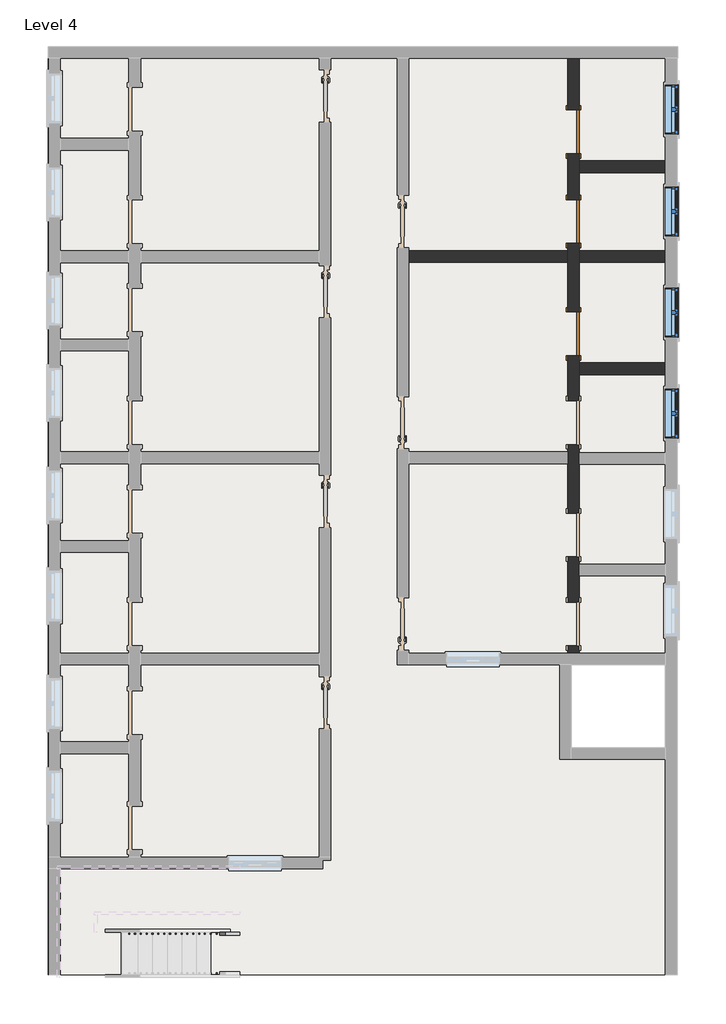
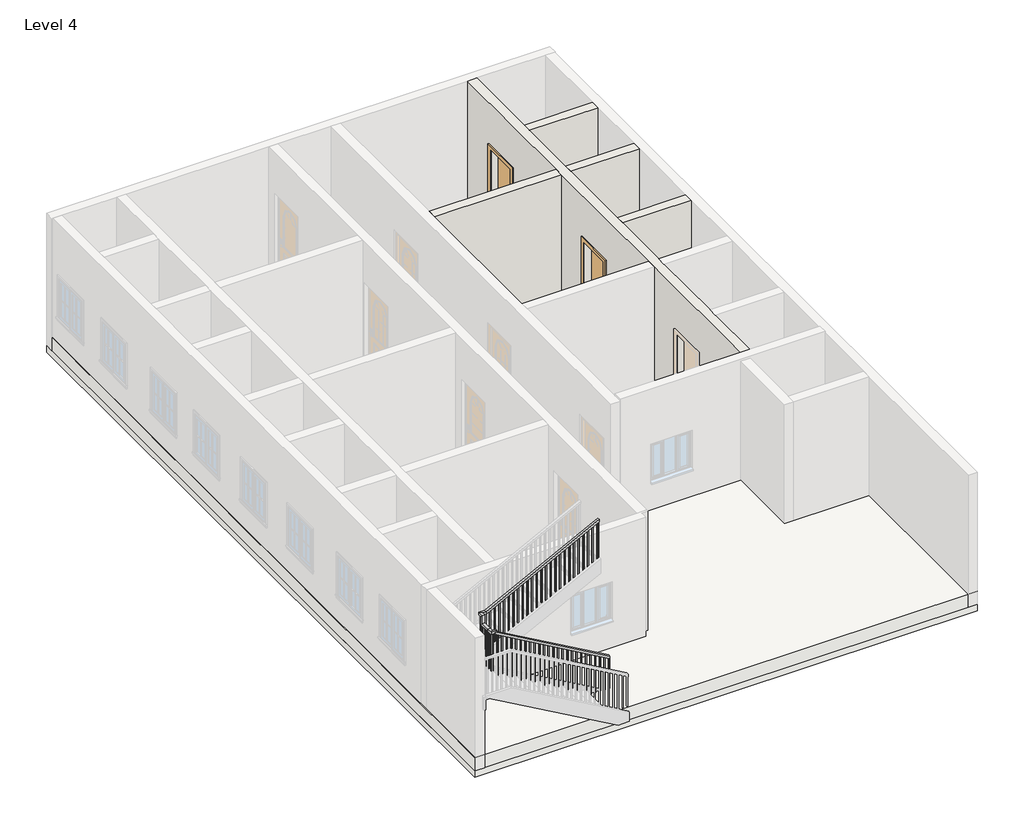
# One storey, part 2 of 4: 5 walls, 4 windows, 3 doors, 1 railing, 1 roof, 1 slab.
"""IFC4 building model written with IfcOpenShell, lengths in millimetres."""

from ifc_helpers import new_model, si_unit, frame, origin, place, context, project, spatial, polyline, outline, extrude, faceted_brep, transform, mapped, element, save
from components import door_53b1b562, window_c29befe5

model = new_model("IFC4")

# Units and contexts
model_context = context("Model", 3, world=origin())
ifc_project = project(units=[si_unit("LENGTHUNIT", "METRE", prefix="MILLI")], contexts=[model_context])

# Site, building, storey
site = spatial("IfcSite", under=ifc_project)
building = spatial("IfcBuilding", under=site)
storey = spatial("IfcBuildingStorey", under=building, Name="Level 4", Elevation=9144.0)

# Doors
placement = place(None, origin())
door_shape = door_53b1b562(model_context)
element("IfcDoor", 1, ObjectType="Single-Flush : 30\" x 80\"", at=placement, inside=storey, context=model_context, shape_type="MappedRepresentation", body=[
    mapped(door_shape, transform((2695.5891134, 6512.9399728, 9144.0), x_axis=(0.0, 1.0, 0.0), y_axis=(-1.0, 0.0, 0.0), z_axis=(0.0, 0.0, 1.0))),
])
element("IfcDoor", 2, ObjectType="Single-Flush : 30\" x 80\"", at=placement, inside=storey, context=model_context, shape_type="MappedRepresentation", body=[
    mapped(door_shape, transform((2695.5891134, 4950.8399728, 9144.0), x_axis=(0.0, 1.0, 0.0), y_axis=(-1.0, 0.0, 0.0), z_axis=(0.0, 0.0, 1.0))),
])
element("IfcDoor", 3, ObjectType="Single-Flush : 30\" x 80\"", at=placement, inside=storey, context=model_context, shape_type="MappedRepresentation", body=[
    mapped(door_shape, transform((2695.5891134, 2995.0399728, 9144.0), x_axis=(0.0, 1.0, 0.0), y_axis=(-1.0, 0.0, 0.0), z_axis=(0.0, 0.0, 1.0))),
])

# Railing
element("IfcRailing", 4, ObjectType="Handrail - Rectangular", at=placement, inside=storey, context=model_context, shape_type="SolidModel", body=[
    faceted_brep([(-3117.2664982, -7482.4600272, 10203.5428571), (-3117.2664982, -7482.4600272, 10145.0339009), (-3117.2664982, -7431.6600272, 10145.0339009), (-3117.2664982, -7431.6600272, 10203.5428571), (-5581.0664982, -7482.4600272, 11611.4285714), (-5631.8664982, -7482.4600272, 11581.9481866), (-5631.8664982, -7431.6600272, 11581.9481866), (-5581.0664982, -7431.6600272, 11611.4285714), (-5581.0664982, -7482.4600272, 11654.9714286), (-5631.8664982, -7482.4600272, 11604.1714286), (-5631.8664982, -7431.6600272, 11604.1714286), (-5581.0664982, -7431.6600272, 11654.9714286), (-5708.0664982, -7482.4600272, 11654.9714286), (-5708.0664982, -7482.4600272, 11604.1714286), (-5657.2664982, -7431.6600272, 11604.1714286), (-5657.2664982, -7431.6600272, 11654.9714286), (-5708.0664982, -7355.4600272, 11654.9714286), (-5708.0664982, -7355.4600272, 11604.1714286), (-5657.2664982, -7355.4600272, 11604.1714286), (-5657.2664982, -7355.4600272, 11654.9714286), (-5708.0664982, -7152.2600272, 11654.9714286), (-5708.0664982, -7101.4600272, 11604.1714286), (-5657.2664982, -7101.4600272, 11604.1714286), (-5657.2664982, -7152.2600272, 11654.9714286), (-5708.0664982, -7152.2600272, 11839.3028571), (-5708.0664982, -7101.4600272, 11788.5028571), (-5657.2664982, -7101.4600272, 11788.5028571), (-5657.2664982, -7152.2600272, 11839.3028571), (-5708.0664982, -7025.2600272, 11839.3028571), (-5708.0664982, -7025.2600272, 11788.5028571), (-5657.2664982, -7076.0600272, 11788.5028571), (-5657.2664982, -7076.0600272, 11839.3028571), (-5581.0664982, -7025.2600272, 11839.3028571), (-5568.769124, -7025.2600272, 11788.5028571), (-5568.769124, -7076.0600272, 11788.5028571), (-5581.0664982, -7076.0600272, 11839.3028571), (-3117.2664982, -7025.2600272, 13106.4), (-3117.2664982, -7076.0600272, 13106.4), (-3117.2664982, -7076.0600272, 13049.2756361), (-3117.2664982, -7025.2600272, 13049.2756361)], [[[0, 1, 2, 3]], [[1, 0, 4, 5]], [[2, 1, 5, 6]], [[3, 2, 6, 7]], [[0, 3, 7, 4]], [[5, 4, 8, 9]], [[6, 5, 9, 10]], [[7, 6, 10, 11]], [[4, 7, 11, 8]], [[9, 8, 12, 13]], [[10, 9, 13, 14]], [[11, 10, 14, 15]], [[8, 11, 15, 12]], [[13, 12, 16, 17]], [[14, 13, 17, 18]], [[15, 14, 18, 19]], [[12, 15, 19, 16]], [[17, 16, 20, 21]], [[18, 17, 21, 22]], [[19, 18, 22, 23]], [[16, 19, 23, 20]], [[21, 20, 24, 25]], [[22, 21, 25, 26]], [[23, 22, 26, 27]], [[20, 23, 27, 24]], [[25, 24, 28, 29]], [[26, 25, 29, 30]], [[27, 26, 30, 31]], [[24, 27, 31, 28]], [[29, 28, 32, 33]], [[30, 29, 33, 34]], [[31, 30, 34, 35]], [[28, 31, 35, 32]], [[36, 37, 38, 39]], [[33, 32, 36, 39]], [[34, 33, 39, 38]], [[35, 34, 38, 37]], [[32, 35, 37, 36]]]),
    extrude(outline(polyline([(13041.1113504, -3133.1414982), (13031.3142076, -3152.1914982), (12046.8571429, -3152.1914982), (12046.8571429, -3133.1414982), (13041.1113504, -3133.1414982)])), frame((0.0, -7060.1850272, 0.0), z_axis=(0.0, 1.0, 0.0), x_axis=(0.0, 0.0, 1.0)), (0.0, 0.0, 1.0), 19.05),
    extrude(outline(polyline([(12988.8599218, -3234.7414982), (12979.062779, -3253.7914982), (12046.8571429, -3253.7914982), (12046.8571429, -3234.7414982), (12988.8599218, -3234.7414982)])), frame((0.0, -7060.1850272, 0.0), z_axis=(0.0, 1.0, 0.0), x_axis=(0.0, 0.0, 1.0)), (0.0, 0.0, 1.0), 19.05),
    extrude(outline(polyline([(12936.6084933, -3336.3414982), (12926.8113504, -3355.3914982), (12046.8571429, -3355.3914982), (12046.8571429, -3336.3414982), (12936.6084933, -3336.3414982)])), frame((0.0, -7060.1850272, 0.0), z_axis=(0.0, 1.0, 0.0), x_axis=(0.0, 0.0, 1.0)), (0.0, 0.0, 1.0), 19.05),
    extrude(outline(polyline([(12884.3570647, -3437.9414982), (12874.5599218, -3456.9914982), (11901.7142857, -3456.9914982), (11901.7142857, -3437.9414982), (12884.3570647, -3437.9414982)])), frame((0.0, -7060.1850272, 0.0), z_axis=(0.0, 1.0, 0.0), x_axis=(0.0, 0.0, 1.0)), (0.0, 0.0, 1.0), 19.05),
    extrude(outline(polyline([(12832.1056361, -3539.5414982), (12822.3084933, -3558.5914982), (11901.7142857, -3558.5914982), (11901.7142857, -3539.5414982), (12832.1056361, -3539.5414982)])), frame((0.0, -7060.1850272, 0.0), z_axis=(0.0, 1.0, 0.0), x_axis=(0.0, 0.0, 1.0)), (0.0, 0.0, 1.0), 19.05),
    extrude(outline(polyline([(12779.8542076, -3641.1414982), (12770.0570647, -3660.1914982), (11756.5714286, -3660.1914982), (11756.5714286, -3641.1414982), (12779.8542076, -3641.1414982)])), frame((0.0, -7060.1850272, 0.0), z_axis=(0.0, 1.0, 0.0), x_axis=(0.0, 0.0, 1.0)), (0.0, 0.0, 1.0), 19.05),
    extrude(outline(polyline([(12727.602779, -3742.7414982), (12717.8056361, -3761.7914982), (11756.5714286, -3761.7914982), (11756.5714286, -3742.7414982), (12727.602779, -3742.7414982)])), frame((0.0, -7060.1850272, 0.0), z_axis=(0.0, 1.0, 0.0), x_axis=(0.0, 0.0, 1.0)), (0.0, 0.0, 1.0), 19.05),
    extrude(outline(polyline([(12675.3513504, -3844.3414982), (12665.5542076, -3863.3914982), (11756.5714286, -3863.3914982), (11756.5714286, -3844.3414982), (12675.3513504, -3844.3414982)])), frame((0.0, -7060.1850272, 0.0), z_axis=(0.0, 1.0, 0.0), x_axis=(0.0, 0.0, 1.0)), (0.0, 0.0, 1.0), 19.05),
    extrude(outline(polyline([(12623.0999218, -3945.9414982), (12613.302779, -3964.9914982), (11756.5714286, -3964.9914982), (11756.5714286, -3945.9414982), (12623.0999218, -3945.9414982)])), frame((0.0, -7060.1850272, 0.0), z_axis=(0.0, 1.0, 0.0), x_axis=(0.0, 0.0, 1.0)), (0.0, 0.0, 1.0), 19.05),
    extrude(outline(polyline([(12570.8484933, -4047.5414982), (12561.0513504, -4066.5914982), (11756.5714286, -4066.5914982), (11756.5714286, -4047.5414982), (12570.8484933, -4047.5414982)])), frame((0.0, -7060.1850272, 0.0), z_axis=(0.0, 1.0, 0.0), x_axis=(0.0, 0.0, 1.0)), (0.0, 0.0, 1.0), 19.05),
    extrude(outline(polyline([(12518.5970647, -4149.1414982), (12508.7999218, -4168.1914982), (11611.4285714, -4168.1914982), (11611.4285714, -4149.1414982), (12518.5970647, -4149.1414982)])), frame((0.0, -7060.1850272, 0.0), z_axis=(0.0, 1.0, 0.0), x_axis=(0.0, 0.0, 1.0)), (0.0, 0.0, 1.0), 19.05),
    extrude(outline(polyline([(12466.3456361, -4250.7414982), (12456.5484933, -4269.7914982), (11611.4285714, -4269.7914982), (11611.4285714, -4250.7414982), (12466.3456361, -4250.7414982)])), frame((0.0, -7060.1850272, 0.0), z_axis=(0.0, 1.0, 0.0), x_axis=(0.0, 0.0, 1.0)), (0.0, 0.0, 1.0), 19.05),
    extrude(outline(polyline([(12414.0942076, -4352.3414982), (12404.2970647, -4371.3914982), (11611.4285714, -4371.3914982), (11611.4285714, -4352.3414982), (12414.0942076, -4352.3414982)])), frame((0.0, -7060.1850272, 0.0), z_axis=(0.0, 1.0, 0.0), x_axis=(0.0, 0.0, 1.0)), (0.0, 0.0, 1.0), 19.05),
    extrude(outline(polyline([(12361.842779, -4453.9414982), (12352.0456361, -4472.9914982), (11466.2857143, -4472.9914982), (11466.2857143, -4453.9414982), (12361.842779, -4453.9414982)])), frame((0.0, -7060.1850272, 0.0), z_axis=(0.0, 1.0, 0.0), x_axis=(0.0, 0.0, 1.0)), (0.0, 0.0, 1.0), 19.05),
    extrude(outline(polyline([(12309.5913504, -4555.5414982), (12299.7942076, -4574.5914982), (11466.2857143, -4574.5914982), (11466.2857143, -4555.5414982), (12309.5913504, -4555.5414982)])), frame((0.0, -7060.1850272, 0.0), z_axis=(0.0, 1.0, 0.0), x_axis=(0.0, 0.0, 1.0)), (0.0, 0.0, 1.0), 19.05),
    extrude(outline(polyline([(12257.3399218, -4657.1414982), (12247.542779, -4676.1914982), (11321.1428571, -4676.1914982), (11321.1428571, -4657.1414982), (12257.3399218, -4657.1414982)])), frame((0.0, -7060.1850272, 0.0), z_axis=(0.0, 1.0, 0.0), x_axis=(0.0, 0.0, 1.0)), (0.0, 0.0, 1.0), 19.05),
    extrude(outline(polyline([(12205.0884933, -4758.7414982), (12195.2913504, -4777.7914982), (11321.1428571, -4777.7914982), (11321.1428571, -4758.7414982), (12205.0884933, -4758.7414982)])), frame((0.0, -7060.1850272, 0.0), z_axis=(0.0, 1.0, 0.0), x_axis=(0.0, 0.0, 1.0)), (0.0, 0.0, 1.0), 19.05),
    extrude(outline(polyline([(12152.8370647, -4860.3414982), (12143.0399218, -4879.3914982), (11321.1428571, -4879.3914982), (11321.1428571, -4860.3414982), (12152.8370647, -4860.3414982)])), frame((0.0, -7060.1850272, 0.0), z_axis=(0.0, 1.0, 0.0), x_axis=(0.0, 0.0, 1.0)), (0.0, 0.0, 1.0), 19.05),
    extrude(outline(polyline([(12100.5856361, -4961.9414982), (12090.7884933, -4980.9914982), (11176.0, -4980.9914982), (11176.0, -4961.9414982), (12100.5856361, -4961.9414982)])), frame((0.0, -7060.1850272, 0.0), z_axis=(0.0, 1.0, 0.0), x_axis=(0.0, 0.0, 1.0)), (0.0, 0.0, 1.0), 19.05),
    extrude(outline(polyline([(12048.3342076, -5063.5414982), (12038.5370647, -5082.5914982), (11176.0, -5082.5914982), (11176.0, -5063.5414982), (12048.3342076, -5063.5414982)])), frame((0.0, -7060.1850272, 0.0), z_axis=(0.0, 1.0, 0.0), x_axis=(0.0, 0.0, 1.0)), (0.0, 0.0, 1.0), 19.05),
    extrude(outline(polyline([(11996.082779, -5165.1414982), (11986.2856361, -5184.1914982), (11030.8571429, -5184.1914982), (11030.8571429, -5165.1414982), (11996.082779, -5165.1414982)])), frame((0.0, -7060.1850272, 0.0), z_axis=(0.0, 1.0, 0.0), x_axis=(0.0, 0.0, 1.0)), (0.0, 0.0, 1.0), 19.05),
    extrude(outline(polyline([(11943.8313504, -5266.7414982), (11934.0342076, -5285.7914982), (11030.8571429, -5285.7914982), (11030.8571429, -5266.7414982), (11943.8313504, -5266.7414982)])), frame((0.0, -7060.1850272, 0.0), z_axis=(0.0, 1.0, 0.0), x_axis=(0.0, 0.0, 1.0)), (0.0, 0.0, 1.0), 19.05),
    extrude(outline(polyline([(11891.5799218, -5368.3414982), (11881.782779, -5387.3914982), (11030.8571429, -5387.3914982), (11030.8571429, -5368.3414982), (11891.5799218, -5368.3414982)])), frame((0.0, -7060.1850272, 0.0), z_axis=(0.0, 1.0, 0.0), x_axis=(0.0, 0.0, 1.0)), (0.0, 0.0, 1.0), 19.05),
    extrude(outline(polyline([(11839.3284933, -5469.9414982), (11829.5313504, -5488.9914982), (10885.7142857, -5488.9914982), (10885.7142857, -5469.9414982), (11839.3284933, -5469.9414982)])), frame((0.0, -7060.1850272, 0.0), z_axis=(0.0, 1.0, 0.0), x_axis=(0.0, 0.0, 1.0)), (0.0, 0.0, 1.0), 19.05),
    extrude(outline(polyline([(11787.0770647, -5571.5414982), (11777.2799218, -5590.5914982), (10885.7142857, -5590.5914982), (10885.7142857, -5571.5414982), (11787.0770647, -5571.5414982)])), frame((0.0, -7060.1850272, 0.0), z_axis=(0.0, 1.0, 0.0), x_axis=(0.0, 0.0, 1.0)), (0.0, 0.0, 1.0), 19.05),
    extrude(outline(polyline([(-5673.1414982, -7161.7850272), (-5692.1914982, -7161.7850272), (-5692.1914982, -7142.7350272), (-5673.1414982, -7142.7350272), (-5673.1414982, -7161.7850272)])), frame((0.0, 0.0, 10740.5714286), z_axis=(0.0, 0.0, 1.0), x_axis=(1.0, 0.0, 0.0)), (0.0, 0.0, 1.0), 863.6),
    extrude(outline(polyline([(-5673.1414982, -7263.3850272), (-5692.1914982, -7263.3850272), (-5692.1914982, -7244.3350272), (-5673.1414982, -7244.3350272), (-5673.1414982, -7263.3850272)])), frame((0.0, 0.0, 10740.5714286), z_axis=(0.0, 0.0, 1.0), x_axis=(1.0, 0.0, 0.0)), (0.0, 0.0, 1.0), 863.6),
    extrude(outline(polyline([(-5673.1414982, -7364.9850272), (-5692.1914982, -7364.9850272), (-5692.1914982, -7345.9350272), (-5673.1414982, -7345.9350272), (-5673.1414982, -7364.9850272)])), frame((0.0, 0.0, 10740.5714286), z_axis=(0.0, 0.0, 1.0), x_axis=(1.0, 0.0, 0.0)), (0.0, 0.0, 1.0), 863.6),
    extrude(outline(polyline([(-5647.7414982, -7447.5350272), (-5647.7414982, -7466.5850272), (-5666.7914982, -7466.5850272), (-5666.7914982, -7447.5350272), (-5647.7414982, -7447.5350272)])), frame((0.0, 0.0, 10740.5714286), z_axis=(0.0, 0.0, 1.0), x_axis=(1.0, 0.0, 0.0)), (0.0, 0.0, 1.0), 863.6),
    extrude(outline(polyline([(11532.9624723, -5546.1414982), (11543.8481866, -5565.1914982), (10595.4285714, -5565.1914982), (10595.4285714, -5546.1414982), (11532.9624723, -5546.1414982)])), frame((0.0, -7466.5850272, 0.0), z_axis=(0.0, 1.0, 0.0), x_axis=(0.0, 0.0, 1.0)), (0.0, 0.0, 1.0), 19.05),
    extrude(outline(polyline([(11474.9053295, -5444.5414982), (11485.7910438, -5463.5914982), (10595.4285714, -5463.5914982), (10595.4285714, -5444.5414982), (11474.9053295, -5444.5414982)])), frame((0.0, -7466.5850272, 0.0), z_axis=(0.0, 1.0, 0.0), x_axis=(0.0, 0.0, 1.0)), (0.0, 0.0, 1.0), 19.05),
    extrude(outline(polyline([(11416.8481866, -5342.9414982), (11427.7339009, -5361.9914982), (10450.2857143, -5361.9914982), (10450.2857143, -5342.9414982), (11416.8481866, -5342.9414982)])), frame((0.0, -7466.5850272, 0.0), z_axis=(0.0, 1.0, 0.0), x_axis=(0.0, 0.0, 1.0)), (0.0, 0.0, 1.0), 19.05),
    extrude(outline(polyline([(11358.7910438, -5241.3414982), (11369.6767581, -5260.3914982), (10450.2857143, -5260.3914982), (10450.2857143, -5241.3414982), (11358.7910438, -5241.3414982)])), frame((0.0, -7466.5850272, 0.0), z_axis=(0.0, 1.0, 0.0), x_axis=(0.0, 0.0, 1.0)), (0.0, 0.0, 1.0), 19.05),
    extrude(outline(polyline([(11300.7339009, -5139.7414982), (11311.6196152, -5158.7914982), (10450.2857143, -5158.7914982), (10450.2857143, -5139.7414982), (11300.7339009, -5139.7414982)])), frame((0.0, -7466.5850272, 0.0), z_axis=(0.0, 1.0, 0.0), x_axis=(0.0, 0.0, 1.0)), (0.0, 0.0, 1.0), 19.05),
    extrude(outline(polyline([(11242.6767581, -5038.1414982), (11253.5624723, -5057.1914982), (10305.1428571, -5057.1914982), (10305.1428571, -5038.1414982), (11242.6767581, -5038.1414982)])), frame((0.0, -7466.5850272, 0.0), z_axis=(0.0, 1.0, 0.0), x_axis=(0.0, 0.0, 1.0)), (0.0, 0.0, 1.0), 19.05),
    extrude(outline(polyline([(11184.6196152, -4936.5414982), (11195.5053295, -4955.5914982), (10305.1428571, -4955.5914982), (10305.1428571, -4936.5414982), (11184.6196152, -4936.5414982)])), frame((0.0, -7466.5850272, 0.0), z_axis=(0.0, 1.0, 0.0), x_axis=(0.0, 0.0, 1.0)), (0.0, 0.0, 1.0), 19.05),
    extrude(outline(polyline([(11126.5624723, -4834.9414982), (11137.4481866, -4853.9914982), (10160.0, -4853.9914982), (10160.0, -4834.9414982), (11126.5624723, -4834.9414982)])), frame((0.0, -7466.5850272, 0.0), z_axis=(0.0, 1.0, 0.0), x_axis=(0.0, 0.0, 1.0)), (0.0, 0.0, 1.0), 19.05),
    extrude(outline(polyline([(11068.5053295, -4733.3414982), (11079.3910438, -4752.3914982), (10160.0, -4752.3914982), (10160.0, -4733.3414982), (11068.5053295, -4733.3414982)])), frame((0.0, -7466.5850272, 0.0), z_axis=(0.0, 1.0, 0.0), x_axis=(0.0, 0.0, 1.0)), (0.0, 0.0, 1.0), 19.05),
    extrude(outline(polyline([(11010.4481866, -4631.7414982), (11021.3339009, -4650.7914982), (10160.0, -4650.7914982), (10160.0, -4631.7414982), (11010.4481866, -4631.7414982)])), frame((0.0, -7466.5850272, 0.0), z_axis=(0.0, 1.0, 0.0), x_axis=(0.0, 0.0, 1.0)), (0.0, 0.0, 1.0), 19.05),
    extrude(outline(polyline([(10952.3910438, -4530.1414982), (10963.2767581, -4549.1914982), (10014.8571429, -4549.1914982), (10014.8571429, -4530.1414982), (10952.3910438, -4530.1414982)])), frame((0.0, -7466.5850272, 0.0), z_axis=(0.0, 1.0, 0.0), x_axis=(0.0, 0.0, 1.0)), (0.0, 0.0, 1.0), 19.05),
    extrude(outline(polyline([(10894.3339009, -4428.5414982), (10905.2196152, -4447.5914982), (10014.8571429, -4447.5914982), (10014.8571429, -4428.5414982), (10894.3339009, -4428.5414982)])), frame((0.0, -7466.5850272, 0.0), z_axis=(0.0, 1.0, 0.0), x_axis=(0.0, 0.0, 1.0)), (0.0, 0.0, 1.0), 19.05),
    extrude(outline(polyline([(10836.2767581, -4326.9414982), (10847.1624723, -4345.9914982), (9869.7142857, -4345.9914982), (9869.7142857, -4326.9414982), (10836.2767581, -4326.9414982)])), frame((0.0, -7466.5850272, 0.0), z_axis=(0.0, 1.0, 0.0), x_axis=(0.0, 0.0, 1.0)), (0.0, 0.0, 1.0), 19.05),
    extrude(outline(polyline([(10778.2196152, -4225.3414982), (10789.1053295, -4244.3914982), (9869.7142857, -4244.3914982), (9869.7142857, -4225.3414982), (10778.2196152, -4225.3414982)])), frame((0.0, -7466.5850272, 0.0), z_axis=(0.0, 1.0, 0.0), x_axis=(0.0, 0.0, 1.0)), (0.0, 0.0, 1.0), 19.05),
    extrude(outline(polyline([(10720.1624723, -4123.7414982), (10731.0481866, -4142.7914982), (9869.7142857, -4142.7914982), (9869.7142857, -4123.7414982), (10720.1624723, -4123.7414982)])), frame((0.0, -7466.5850272, 0.0), z_axis=(0.0, 1.0, 0.0), x_axis=(0.0, 0.0, 1.0)), (0.0, 0.0, 1.0), 19.05),
    extrude(outline(polyline([(10662.1053295, -4022.1414982), (10672.9910438, -4041.1914982), (9724.5714286, -4041.1914982), (9724.5714286, -4022.1414982), (10662.1053295, -4022.1414982)])), frame((0.0, -7466.5850272, 0.0), z_axis=(0.0, 1.0, 0.0), x_axis=(0.0, 0.0, 1.0)), (0.0, 0.0, 1.0), 19.05),
    extrude(outline(polyline([(10604.0481866, -3920.5414982), (10614.9339009, -3939.5914982), (9724.5714286, -3939.5914982), (9724.5714286, -3920.5414982), (10604.0481866, -3920.5414982)])), frame((0.0, -7466.5850272, 0.0), z_axis=(0.0, 1.0, 0.0), x_axis=(0.0, 0.0, 1.0)), (0.0, 0.0, 1.0), 19.05),
    extrude(outline(polyline([(10545.9910438, -3818.9414982), (10556.8767581, -3837.9914982), (9579.4285714, -3837.9914982), (9579.4285714, -3818.9414982), (10545.9910438, -3818.9414982)])), frame((0.0, -7466.5850272, 0.0), z_axis=(0.0, 1.0, 0.0), x_axis=(0.0, 0.0, 1.0)), (0.0, 0.0, 1.0), 19.05),
    extrude(outline(polyline([(10487.9339009, -3717.3414982), (10498.8196152, -3736.3914982), (9579.4285714, -3736.3914982), (9579.4285714, -3717.3414982), (10487.9339009, -3717.3414982)])), frame((0.0, -7466.5850272, 0.0), z_axis=(0.0, 1.0, 0.0), x_axis=(0.0, 0.0, 1.0)), (0.0, 0.0, 1.0), 19.05),
    extrude(outline(polyline([(10429.8767581, -3615.7414982), (10440.7624723, -3634.7914982), (9579.4285714, -3634.7914982), (9579.4285714, -3615.7414982), (10429.8767581, -3615.7414982)])), frame((0.0, -7466.5850272, 0.0), z_axis=(0.0, 1.0, 0.0), x_axis=(0.0, 0.0, 1.0)), (0.0, 0.0, 1.0), 19.05),
    extrude(outline(polyline([(10371.8196152, -3514.1414982), (10382.7053295, -3533.1914982), (9434.2857143, -3533.1914982), (9434.2857143, -3514.1414982), (10371.8196152, -3514.1414982)])), frame((0.0, -7466.5850272, 0.0), z_axis=(0.0, 1.0, 0.0), x_axis=(0.0, 0.0, 1.0)), (0.0, 0.0, 1.0), 19.05),
    extrude(outline(polyline([(10313.7624723, -3412.5414982), (10324.6481866, -3431.5914982), (9434.2857143, -3431.5914982), (9434.2857143, -3412.5414982), (10313.7624723, -3412.5414982)])), frame((0.0, -7466.5850272, 0.0), z_axis=(0.0, 1.0, 0.0), x_axis=(0.0, 0.0, 1.0)), (0.0, 0.0, 1.0), 19.05),
    extrude(outline(polyline([(10255.7053295, -3310.9414982), (10266.5910438, -3329.9914982), (9289.1428571, -3329.9914982), (9289.1428571, -3310.9414982), (10255.7053295, -3310.9414982)])), frame((0.0, -7466.5850272, 0.0), z_axis=(0.0, 1.0, 0.0), x_axis=(0.0, 0.0, 1.0)), (0.0, 0.0, 1.0), 19.05),
    extrude(outline(polyline([(10197.6481866, -3209.3414982), (10208.5339009, -3228.3914982), (9289.1428571, -3228.3914982), (9289.1428571, -3209.3414982), (10197.6481866, -3209.3414982)])), frame((0.0, -7466.5850272, 0.0), z_axis=(0.0, 1.0, 0.0), x_axis=(0.0, 0.0, 1.0)), (0.0, 0.0, 1.0), 19.05),
    extrude(outline(polyline([(-5673.1414982, -7060.1850272), (-5692.1914982, -7060.1850272), (-5692.1914982, -7041.1350272), (-5673.1414982, -7041.1350272), (-5673.1414982, -7060.1850272)])), frame((0.0, 0.0, 10740.5714286), z_axis=(0.0, 0.0, 1.0), x_axis=(1.0, 0.0, 0.0)), (0.0, 0.0, 1.0), 1047.9314286),
    extrude(outline(polyline([(-5673.1414982, -7447.5350272), (-5673.1414982, -7466.5850272), (-5692.1914982, -7466.5850272), (-5692.1914982, -7447.5350272), (-5673.1414982, -7447.5350272)])), frame((0.0, 0.0, 10740.5714286), z_axis=(0.0, 0.0, 1.0), x_axis=(1.0, 0.0, 0.0)), (0.0, 0.0, 1.0), 863.6),
    extrude(outline(polyline([(13049.2756361, -3117.2664982), (13039.4784933, -3136.3164982), (12046.8571429, -3136.3164982), (12046.8571429, -3117.2664982), (13049.2756361, -3117.2664982)])), frame((0.0, -7060.1850272, 0.0), z_axis=(0.0, 1.0, 0.0), x_axis=(0.0, 0.0, 1.0)), (0.0, 0.0, 1.0), 19.05),
    extrude(outline(polyline([(10145.0339009, -3117.2664982), (10155.9196152, -3136.3164982), (9289.1428571, -3136.3164982), (9289.1428571, -3117.2664982), (10145.0339009, -3117.2664982)])), frame((0.0, -7466.5850272, 0.0), z_axis=(0.0, 1.0, 0.0), x_axis=(0.0, 0.0, 1.0)), (0.0, 0.0, 1.0), 19.05),
])

# Roof
element("IfcRoof", 5, ObjectType="Generic - 12\"", at=placement, inside=storey, context=model_context, shape_type="SweptSolid", body=[
    extrude(outline(polyline([(-6461.1108866, -8168.2600272), (-6461.1108866, 7998.8399728), (4498.9891134, 7998.8399728), (4498.9891134, -8168.2600272), (-6461.1108866, -8168.2600272)]), holes=[polyline([(4295.7891134, -2770.7600272), (2657.4891134, -2770.7600272), (2657.4891134, -4218.5600272), (4295.7891134, -4218.5600272), (4295.7891134, -2770.7600272)])]), frame((0.0, 0.0, 9144.0), z_axis=(0.0, 0.0, 1.0), x_axis=(1.0, 0.0, 0.0)), (0.0, 0.0, 1.0), 304.8),
])

# Slab
element("IfcSlab", 6, ObjectType="Generic - 12\"", at=placement, inside=storey, context=model_context, shape_type="SweptSolid", body=[
    extrude(outline(polyline([(4498.9891134, 7998.8399728), (4498.9891134, -8168.2600272), (-6461.1108866, -8168.2600272), (-6461.1108866, 7998.8399728), (4498.9891134, 7998.8399728)]), holes=[polyline([(4295.7891134, -2770.7600272), (2657.4891134, -2770.7600272), (2657.4891134, -4218.5600272), (4295.7891134, -4218.5600272), (4295.7891134, -2770.7600272)])]), frame((0.0, 0.0, 8991.6), z_axis=(0.0, 0.0, 1.0), x_axis=(1.0, 0.0, 0.0)), (0.0, 0.0, 1.0), 152.4),
])

# Walls
element("IfcWall", 7, ObjectType="4.5\" p", at=placement, inside=storey, context=model_context, shape_type="Brep", body=[
    faceted_brep([(2593.9891134, -2440.5600272, 11176.0), (2593.9891134, -2440.5600272, 9144.0), (2593.9891134, -2567.5600272, 9144.0), (2593.9891134, -2567.5600272, 12192.0), (2593.9891134, 734.4399728, 12192.0), (2593.9891134, 937.6399728, 12192.0), (2593.9891134, 4239.6399728, 12192.0), (2593.9891134, 4442.8399728, 12192.0), (2593.9891134, 7795.6399728, 12192.0), (2593.9891134, 7795.6399728, 9144.0), (2593.9891134, 6893.9399728, 9144.0), (2593.9891134, 6893.9399728, 11176.0), (2593.9891134, 6131.9399728, 11176.0), (2593.9891134, 6131.9399728, 9144.0), (2593.9891134, 5331.8399728, 9144.0), (2593.9891134, 5331.8399728, 11176.0), (2593.9891134, 4569.8399728, 11176.0), (2593.9891134, 4569.8399728, 9144.0), (2593.9891134, 4442.8399728, 9144.0), (2593.9891134, 4239.6399728, 9144.0), (2593.9891134, 3376.0399728, 9144.0), (2593.9891134, 3376.0399728, 11176.0), (2593.9891134, 2614.0399728, 11176.0), (2593.9891134, 2614.0399728, 9144.0), (2593.9891134, 1826.6399728, 9144.0), (2593.9891134, 1826.6399728, 11176.0), (2593.9891134, 1064.6399728, 11176.0), (2593.9891134, 1064.6399728, 9144.0), (2593.9891134, 937.6399728, 9144.0), (2593.9891134, 734.4399728, 9144.0), (2593.9891134, -129.1600272, 9144.0), (2593.9891134, -129.1600272, 11176.0), (2593.9891134, -891.1600272, 11176.0), (2593.9891134, -891.1600272, 9144.0), (2593.9891134, -1678.5600272, 9144.0), (2593.9891134, -1678.5600272, 11176.0), (2797.1891134, -2567.5600272, 9144.0), (2797.1891134, -2440.5600272, 9144.0), (2797.1891134, -2440.5600272, 11176.0), (2797.1891134, -1678.5600272, 11176.0), (2797.1891134, -1678.5600272, 9144.0), (2797.1891134, -1221.3600272, 9144.0), (2797.1891134, -1018.1600272, 9144.0), (2797.1891134, -891.1600272, 9144.0), (2797.1891134, -891.1600272, 11176.0), (2797.1891134, -129.1600272, 11176.0), (2797.1891134, -129.1600272, 9144.0), (2797.1891134, 721.7399728, 9144.0), (2797.1891134, 924.9399728, 9144.0), (2797.1891134, 1064.6399728, 9144.0), (2797.1891134, 1064.6399728, 11176.0), (2797.1891134, 1826.6399728, 11176.0), (2797.1891134, 1826.6399728, 9144.0), (2797.1891134, 2283.8399728, 9144.0), (2797.1891134, 2487.0399728, 9144.0), (2797.1891134, 2614.0399728, 9144.0), (2797.1891134, 2614.0399728, 11176.0), (2797.1891134, 3376.0399728, 11176.0), (2797.1891134, 3376.0399728, 9144.0), (2797.1891134, 4239.6399728, 9144.0), (2797.1891134, 4442.8399728, 9144.0), (2797.1891134, 4569.8399728, 9144.0), (2797.1891134, 4569.8399728, 11176.0), (2797.1891134, 5331.8399728, 11176.0), (2797.1891134, 5331.8399728, 9144.0), (2797.1891134, 5801.7399728, 9144.0), (2797.1891134, 6004.9399728, 9144.0), (2797.1891134, 6131.9399728, 9144.0), (2797.1891134, 6131.9399728, 11176.0), (2797.1891134, 6893.9399728, 11176.0), (2797.1891134, 6893.9399728, 9144.0), (2797.1891134, 7795.6399728, 9144.0), (2797.1891134, 7795.6399728, 12192.0), (2797.1891134, 6004.9399728, 12192.0), (2797.1891134, 5801.7399728, 12192.0), (2797.1891134, 4442.8399728, 12192.0), (2797.1891134, 4239.6399728, 12192.0), (2797.1891134, 2487.0399728, 12192.0), (2797.1891134, 2283.8399728, 12192.0), (2797.1891134, 924.9399728, 12192.0), (2797.1891134, 721.7399728, 12192.0), (2797.1891134, -1018.1600272, 12192.0), (2797.1891134, -1221.3600272, 12192.0), (2797.1891134, -2567.5600272, 12192.0)], [[[0, 1, 2, 3, 4, 5, 6, 7, 8, 9, 10, 11, 12, 13, 14, 15, 16, 17, 18, 19, 20, 21, 22, 23, 24, 25, 26, 27, 28, 29, 30, 31, 32, 33, 34, 35]], [[36, 37, 38, 39, 40, 41, 42, 43, 44, 45, 46, 47, 48, 49, 50, 51, 52, 53, 54, 55, 56, 57, 58, 59, 60, 61, 62, 63, 64, 65, 66, 67, 68, 69, 70, 71, 72, 73, 74, 75, 76, 77, 78, 79, 80, 81, 82, 83]], [[71, 70, 10, 9]], [[67, 66, 65, 64, 14, 13]], [[61, 60, 59, 58, 20, 19, 18, 17]], [[55, 54, 53, 52, 24, 23]], [[30, 29, 28, 27, 49, 48, 47, 46]], [[34, 33, 43, 42, 41, 40]], [[2, 1, 37, 36]], [[8, 7, 6, 5, 4, 3, 83, 82, 81, 80, 79, 78, 77, 76, 75, 74, 73, 72]], [[9, 8, 72, 71]], [[3, 2, 36, 83]], [[11, 10, 70, 69]], [[12, 11, 69, 68]], [[13, 12, 68, 67]], [[15, 14, 64, 63]], [[16, 15, 63, 62]], [[17, 16, 62, 61]], [[21, 20, 58, 57]], [[22, 21, 57, 56]], [[23, 22, 56, 55]], [[25, 24, 52, 51]], [[26, 25, 51, 50]], [[27, 26, 50, 49]], [[44, 43, 33, 32]], [[45, 44, 32, 31]], [[46, 45, 31, 30]], [[38, 37, 1, 0]], [[39, 38, 0, 35]], [[40, 39, 35, 34]]]),
])
element("IfcWall", 8, ObjectType="4.5\" p", at=placement, inside=storey, context=model_context, shape_type="SweptSolid", body=[
    extrude(outline(polyline([(4295.7891134, 5801.7399728), (2797.1891134, 5801.7399728), (2797.1891134, 6004.9399728), (4295.7891134, 6004.9399728), (4295.7891134, 5801.7399728)])), frame((0.0, 0.0, 9144.0), z_axis=(0.0, 0.0, 1.0), x_axis=(1.0, 0.0, 0.0)), (0.0, 0.0, 1.0), 3048.0),
])
element("IfcWall", 9, ObjectType="4.5\" p", at=placement, inside=storey, context=model_context, shape_type="SweptSolid", body=[
    extrude(outline(polyline([(4295.7891134, 4239.6399728), (2797.1891134, 4239.6399728), (2797.1891134, 4442.8399728), (4295.7891134, 4442.8399728), (4295.7891134, 4239.6399728)])), frame((0.0, 0.0, 9144.0), z_axis=(0.0, 0.0, 1.0), x_axis=(1.0, 0.0, 0.0)), (0.0, 0.0, 1.0), 3048.0),
])
element("IfcWall", 10, ObjectType="4.5\" p", at=placement, inside=storey, context=model_context, shape_type="SweptSolid", body=[
    extrude(outline(polyline([(4295.7891134, 2283.8399728), (2797.1891134, 2283.8399728), (2797.1891134, 2487.0399728), (4295.7891134, 2487.0399728), (4295.7891134, 2283.8399728)])), frame((0.0, 0.0, 9144.0), z_axis=(0.0, 0.0, 1.0), x_axis=(1.0, 0.0, 0.0)), (0.0, 0.0, 1.0), 3048.0),
])
element("IfcWall", 11, ObjectType="4.5\" p", at=placement, inside=storey, context=model_context, shape_type="SweptSolid", body=[
    extrude(outline(polyline([(2593.9891134, 4239.6399728), (-174.6108866, 4239.6399728), (-174.6108866, 4442.8399728), (2593.9891134, 4442.8399728), (2593.9891134, 4239.6399728)])), frame((0.0, 0.0, 9144.0), z_axis=(0.0, 0.0, 1.0), x_axis=(1.0, 0.0, 0.0)), (0.0, 0.0, 1.0), 3048.0),
])

# Windows
window_shape = window_c29befe5(model_context)
element("IfcWindow", 12, ObjectType="Window-Casement-Double : 34\" x 36\"", at=placement, inside=storey, context=model_context, shape_type="MappedRepresentation", body=[
    mapped(window_shape, transform((4397.3891134, 1604.3899728, 9144.0), x_axis=(0.0, -1.0, 0.0), y_axis=(1.0, 0.0, 0.0), z_axis=(0.0, 0.0, 1.0))),
])
element("IfcWindow", 13, ObjectType="Window-Casement-Double : 34\" x 36\"", at=placement, inside=storey, context=model_context, shape_type="MappedRepresentation", body=[
    mapped(window_shape, transform((4397.3891134, 3363.3399728, 9144.0), x_axis=(0.0, -1.0, 0.0), y_axis=(1.0, 0.0, 0.0), z_axis=(0.0, 0.0, 1.0))),
])
element("IfcWindow", 14, ObjectType="Window-Casement-Double : 34\" x 36\"", at=placement, inside=storey, context=model_context, shape_type="MappedRepresentation", body=[
    mapped(window_shape, transform((4397.3891134, 5122.2899728, 9144.0), x_axis=(0.0, -1.0, 0.0), y_axis=(1.0, 0.0, 0.0), z_axis=(0.0, 0.0, 1.0))),
])
element("IfcWindow", 15, ObjectType="Window-Casement-Double : 34\" x 36\"", at=placement, inside=storey, context=model_context, shape_type="MappedRepresentation", body=[
    mapped(window_shape, transform((4397.3891134, 6900.2899728, 9144.0), x_axis=(0.0, -1.0, 0.0), y_axis=(1.0, 0.0, 0.0), z_axis=(0.0, 0.0, 1.0))),
])

save(model, "model.ifc")

# Revit data of these elements
# Type "Single-Flush : 30\" x 80\""
#   Type Mark = "5"
#   Construction Type Id = "MDOOR"
#   Assembly Code = "C1020"
#   Analytic Construction = "Metal"
#   Thickness = 0' - 2"
#   Heat Transfer Coefficient (U) = 0.651978 BTU/(h·ft²·°F)
#   Height = 6' - 8"
#   Trim Projection Ext = 0' - 1"
#   Trim Projection Int = 0' - 1"
#   Trim Width = 0' - 3"
#   Width = 2' - 6"
#   Define Thermal Properties by = 1
#   Define Thermal Properties by = 1
#   Door Material = Door - Panel
#   Frame Material = Door - Frame
#   Visual Light Transmittance = 0
#   Solar Heat Gain Coefficient = 0
#   Function = (empty or 0)
#   Wall Closure = (empty or 0)
# Type "Handrail - Rectangular"
#   Assembly Code = "C2010400"
#   built-in parameter 1008612 = 0.0416667 (stored number, unit not read)
#   built-in parameter 1008611 = 0.0416667 (stored number, unit not read)
#   built-in parameter 1008609 = 0.333333 (stored number, unit not read)
#   built-in parameter 1008604 = 0.166667 (stored number, unit not read)
#   built-in parameter 1008603 = 0.166667 (stored number, unit not read)
#   Railing Height = 3' - 0"
#   built-in parameter 1008630 = 2
#   built-in parameter 1008610 = 2
#   built-in parameter 1008618 = Baluster - Square : 3/4"
# Type "Generic - 12\""
#   Assembly Code = "B1020"
#   Layers, outside or top first: 1' - 0" no material (function 1)
# Type "Generic - 12\""
#   Assembly Code = "B1010"
#   Function = 0
#   Layers, outside or top first: 0' - 6" no material (function 1)
# Type "4.5\" p"
#   Assembly Code = "B2010"
#   Layers, outside or top first: 0' - 8" no material (function 1)
# Type "Window-Casement-Double : 34\" x 36\""
#   Type Mark = "14"
#   Fire Rating = "0.5h"
#   Assembly Code = "B2020100"
#   Analytic Construction = "Double glazing - domestic"
#   Frame Extension [instance default] = 0' - 0 1/4"
#   Window Inset [instance default] = 0' - 0"
#   Wall Thickness [instance default] = 0' - 6"
#   Interior Wall Closure [instance default] = 0' - 2 1/4"
#   Half Width = 1' - 5"
#   Visual Light Transmittance = 0.81
#   Thermal Resistance (R) = 1.8146 (h·ft²·°F)/BTU
#   Solar Heat Gain Coefficient = 0.76
#   Rough Width = 2' - 10 1/2"
#   Rough Height = 3' - 0 1/2"
#   Height = 3' - 0"
#   Heat Transfer Coefficient (U) = 0.5511 BTU/(h·ft²·°F)
#   Exterior Wall Closure [instance default] = 0' - 1 1/4"
#   Extension Jamb [instance default] = 0' - 2 1/4"
#   Default Sill Height = 3' - 0"
#   Width = 2' - 10"
#   Define Thermal Properties by = 0
#   Muntin Visibility = yes
#   Interior Trim Visibility [instance default] = yes
#   Exterior Trim Visibility [instance default] = yes
#   Extension Jamb Visibility [instance default] = yes
#   Interior Trim Material = Wood - Stained
#   Muntin Pattern = Muntin Pattern_2x2 : Muntin Pattern_2x2
#   Interior Trim = Trim-Window-Interior-Flat : Picture Frame
#   Interior Frame Material = Wood - Stained
#   Glass Panel Material = Glass
#   Exterior Trim Material = Clad - White
#   Exterior Trim = Trim-Window-Exterior-Flat : with Sill
#   Exterior Frame Material = Clad - White
#   Wall Closure = (empty or 0)
# Elements 1, 2, 3 (IfcDoor, "Single-Flush : 30\" x 80\"")
#   Phase Created = New Construction
#   Materials on its faces: "Door - Frame", "Door - Panel"
# Element 4 (IfcRailing, "Handrail - Rectangular")
#   Phase Created = New Construction
# Element 5 (IfcRoof, "Generic - 12\"")
#   built-in parameter 1001705 = 31 (stored number, unit not read)
#   built-in parameter 1001710 = 33615
#   Phase Created = New Construction
#   Materials on its faces: "Default Roof", "Grass", "Earth"
# Element 6 (IfcSlab, "Generic - 12\"")
#   Height Offset From Level = 0' - 0"
#   Phase Created = New Construction
#   Materials on its faces: "Default Floor", "Earth", "Wood - Stained", "Doors - Glazing Bars"
# Elements 7, 8, 9, 10, 11 (IfcWall, "4.5\" p")
#   Top Offset = 0' - 0"
#   Base Offset = 0' - 0"
#   wall height = 10' - 0"
#   Phase Created = New Construction
#   Base Constraint = Level 4
#   Top Constraint = Level 5
#   Materials on its faces: "Default Wall"
# Element 12 (IfcWindow, "Window-Casement-Double : 34\" x 36\"")
#   Mark = "59"
#   Window Inset = 0' - 0"
#   Interior Wall Closure = 0' - 2 1/4"
#   Frame Extension = 0' - 0 1/4"
#   Exterior Wall Closure = 0' - 1 1/4"
#   Interior Trim Visibility = yes
#   Exterior Trim Visibility = yes
#   Phase Created = New Construction
#   Materials on its faces: "Wood - Stained", "Glass", "Clad - White"
# Element 13 (IfcWindow, "Window-Casement-Double : 34\" x 36\"")
#   Mark = "60"
#   Window Inset = 0' - 0"
#   Interior Wall Closure = 0' - 2 1/4"
#   Frame Extension = 0' - 0 1/4"
#   Exterior Wall Closure = 0' - 1 1/4"
#   Interior Trim Visibility = yes
#   Exterior Trim Visibility = yes
#   Phase Created = New Construction
#   Materials on its faces: "Wood - Stained", "Glass", "Clad - White"
# Element 14 (IfcWindow, "Window-Casement-Double : 34\" x 36\"")
#   Mark = "61"
#   Window Inset = 0' - 0"
#   Interior Wall Closure = 0' - 2 1/4"
#   Frame Extension = 0' - 0 1/4"
#   Exterior Wall Closure = 0' - 1 1/4"
#   Interior Trim Visibility = yes
#   Exterior Trim Visibility = yes
#   Phase Created = New Construction
#   Materials on its faces: "Wood - Stained", "Glass", "Clad - White"
# Element 15 (IfcWindow, "Window-Casement-Double : 34\" x 36\"")
#   Mark = "62"
#   Window Inset = 0' - 0"
#   Interior Wall Closure = 0' - 2 1/4"
#   Frame Extension = 0' - 0 1/4"
#   Exterior Wall Closure = 0' - 1 1/4"
#   Interior Trim Visibility = yes
#   Exterior Trim Visibility = yes
#   Phase Created = New Construction
#   Materials on its faces: "Wood - Stained", "Glass", "Clad - White"
# Materials
#   "Door - Panel": class "Wood", colour RGB 210 159 95, transparency 0, Cost = 0
#   "Door - Frame": colour RGB 118 70 51, transparency 0, Cost = 0
#   "Wood - Stained": class "Wood", colour RGB 224 178 126, transparency 0, Cost = 0
#   "Glass": class "Glass", colour RGB 0 128 192, transparency 0.75, Description = "Soda Lime Glass", Cost = 0
#   "Clad - White": class "Wood", colour RGB 242 242 238, transparency 0, Cost = 0
#   "Default Roof": colour RGB 88 101 114, transparency 0, Cost = 0
#   "Grass": class "Generic", colour RGB 104 137 66, transparency 0, Description = "Physical material.", Cost = 0
#   "Earth": class "Generic", colour RGB 97 75 62, transparency 0, Description = "Soil", Cost = 0
#   "Default Floor": colour RGB 128 128 128, transparency 0, Cost = 0
#   "Doors - Glazing Bars": colour RGB 158 107 65, transparency 0
#   "Default Wall": colour RGB 128 128 128, transparency 0, Cost = 0
